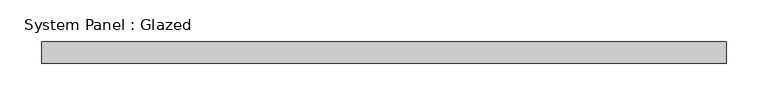
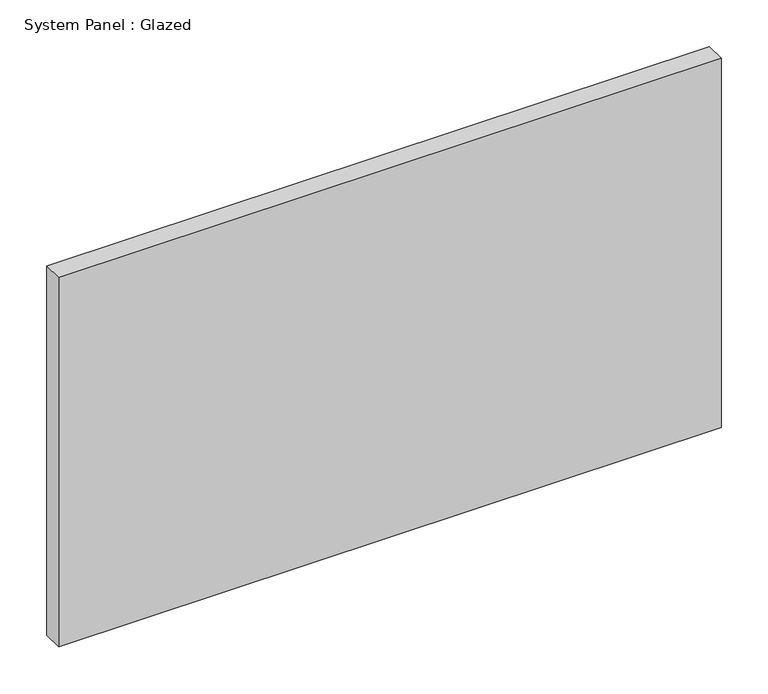
"""IFC4 building model written with IfcOpenShell, lengths in millimetres: plate geometry, System Panel : Glazed."""

from ifc_helpers import new_model, si_unit, origin, origin_with_axes, place, context, project, spatial, polyline, outline, extrude, source, transform, mapped, element, save


def system_panel_glazed_5d767005(model_context):
    return source(origin(), model_context, "Body", "SweptSolid", [
        extrude(outline(polyline([(409.575, 19.05), (-409.575, 19.05), (-409.575, 44.45), (409.575, 44.45), (409.575, 19.05)])), origin_with_axes(), (0.0, 0.0, 1.0), 482.7326807),
    ])


if __name__ == "__main__":
    model = new_model("IFC4")
    model_context = context("Model", 3, world=origin())
    ifc_project = project(units=[si_unit("LENGTHUNIT", "METRE", prefix="MILLI")], contexts=[model_context])
    site = spatial("IfcSite", under=ifc_project)
    building = spatial("IfcBuilding", under=site)
    placement = place(None, origin())
    system_panel_glazed_shape = system_panel_glazed_5d767005(model_context)
    element("IfcPlate", 1, ObjectType="System Panel : Glazed", at=placement, inside=building, context=model_context, shape_type="MappedRepresentation", body=[
        mapped(system_panel_glazed_shape, transform((0.0, 0.0, 0.0), x_axis=(1.0, 0.0, 0.0), y_axis=(0.0, 1.0, 0.0), z_axis=(0.0, 0.0, 1.0))),
    ])
    save(model, "model.ifc")

# Revit data of these elements
# Type "System Panel : Glazed"
#   Construction Type Id = "GSP4R"
#   Analytic Construction = "1/8 in Pilkington single glazing"
#   Visual Light Transmittance = 0.9
#   Solar Heat Gain Coefficient = 0.86
#   Heat Transfer Coefficient (U) = 1.18115 BTU/(h·ft²·°F)
#   Define Thermal Properties by = 1
# Element 1 (IfcPlate, "System Panel : Glazed")
#   Materials on its faces: "Glass"
# Materials
#   "Glass": class "Glass", colour RGB 0 128 192, transparency 0.75, Description = "Soda Lime Glass", Cost = 0
